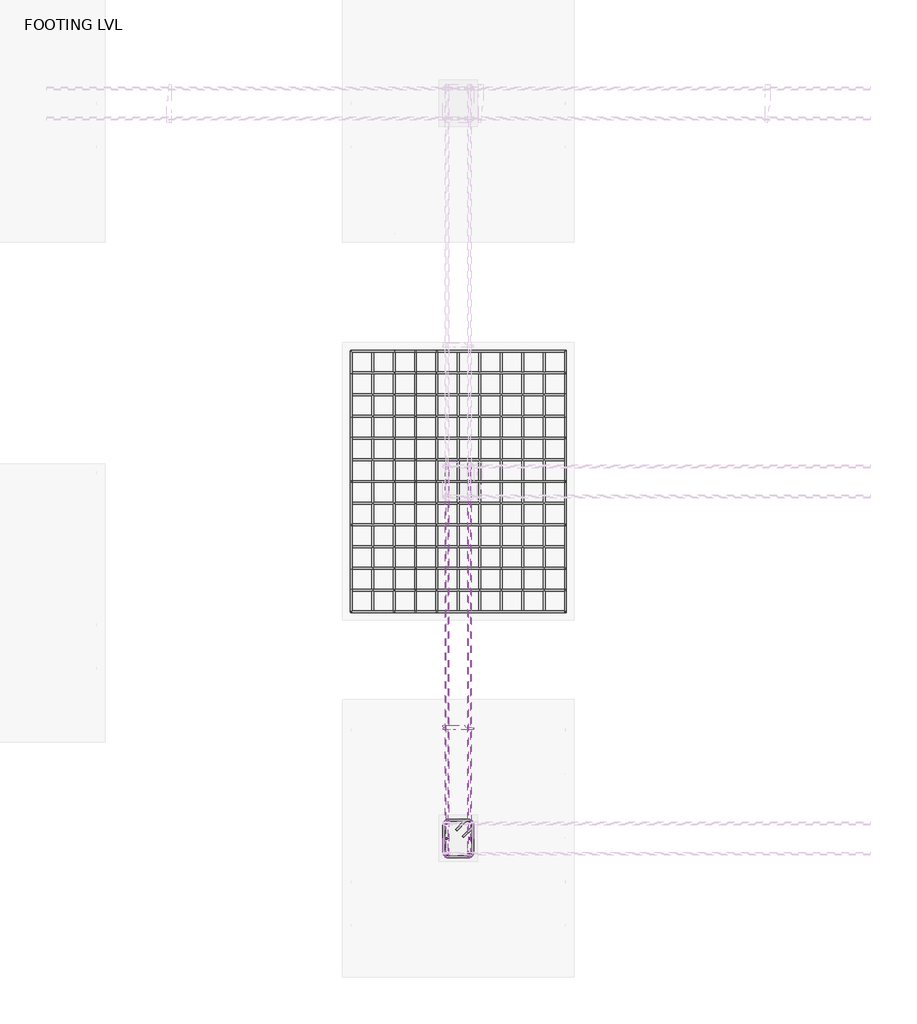
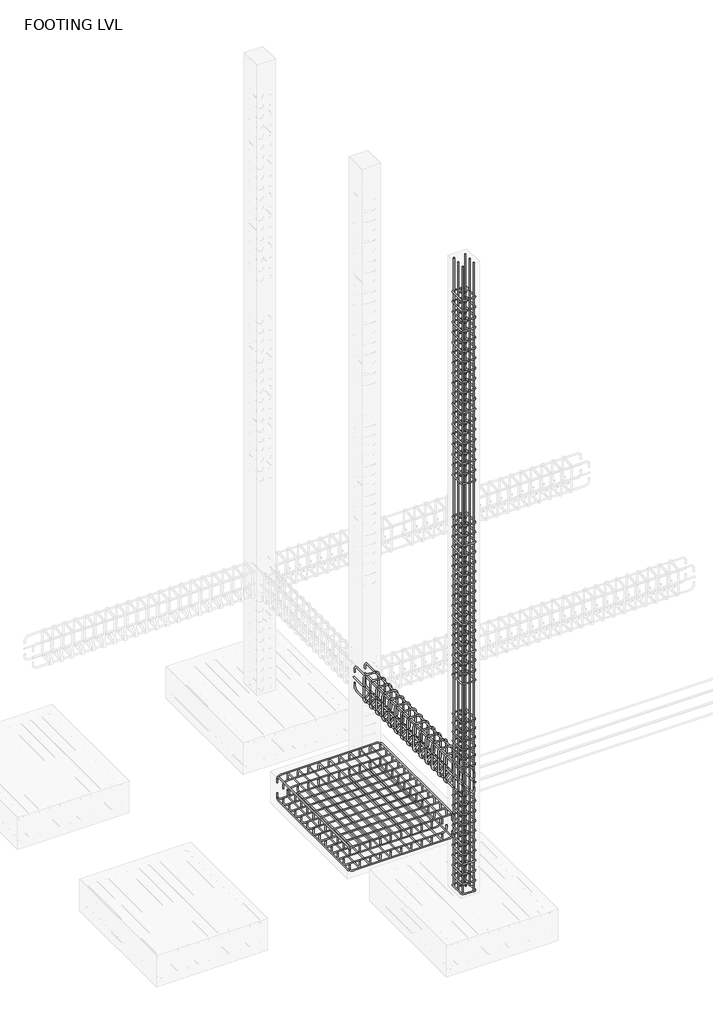
# One storey, part 3 of 16: 21 reinforcing bars.
"""IFC4 building model written with IfcOpenShell, lengths in millimetres."""

from ifc_helpers import new_model, si_unit, point, frame, origin, place, context, project, spatial, polyline, circle_curve, trimmed, segment, composite_curve, source, transform, mapped, element, save
from ifc_brep_helpers import swept_disk

model = new_model("IFC4")

# Units and contexts
model_context = context("Model", 3, world=origin())
ifc_project = project(units=[si_unit("LENGTHUNIT", "METRE", prefix="MILLI")], contexts=[model_context])

# Site, building, storey
site = spatial("IfcSite", under=ifc_project)
building = spatial("IfcBuilding", under=site)
storey = spatial("IfcBuildingStorey", under=building, Name="FOOTING LVL", Elevation=-1828.8)

# Reinforcing bars
placement = place(None, origin())
reinforcing_bar_shape = source(origin(), model_context, "Body", "SolidModel", [
    swept_disk(composite_curve([segment(polyline([(-10315.1165072, 2869.2372759, -2134.39375), (-10315.1165072, 2869.2372759, -2185.19375)]), True, "CONTINUOUS"), segment(trimmed(circle_curve(frame((-10270.6665072, 2869.2372759, -2185.19375), z_axis=(0.0, -1.0, 0.0), x_axis=(-44.45000000000073, 0.0, 0.0)), 44.45), [point((-10315.1165072, 2869.2372759, -2185.19375))], [point((-10270.6665072, 2869.2372759, -2229.64375))], True, "CARTESIAN"), True, "CONTINUOUS"), segment(polyline([(-10270.6665072, 2869.2372759, -2229.64375), (-8948.2790072, 2869.2372759, -2229.64375)]), True, "CONTINUOUS"), segment(trimmed(circle_curve(frame((-8948.2790072, 2869.2372759, -2185.19375), z_axis=(0.0, -1.0, 0.0), x_axis=(0.0, 0.0, -44.45000000000027)), 44.45), [point((-8948.2790072, 2869.2372759, -2229.64375))], [point((-8903.8290072, 2869.2372759, -2185.19375))], True, "CARTESIAN"), True, "CONTINUOUS"), segment(polyline([(-8903.8290072, 2869.2372759, -2185.19375), (-8903.8290072, 2869.2372759, -2134.39375)]), True, "CONTINUOUS")], self_intersect=False), 6.35),
])
element("IfcReinforcingBar", 1, at=placement, inside=storey, context=model_context, shape_type="MappedRepresentation", body=[
    mapped(reinforcing_bar_shape, transform((0.0, 0.0, 0.0), x_axis=(1.0, 0.0, 0.0), y_axis=(0.0, 1.0, 0.0), z_axis=(0.0, 0.0, 1.0))),
    mapped(reinforcing_bar_shape, transform((0.0, 143.0072917, 0.0), x_axis=(1.0, 0.0, 0.0), y_axis=(0.0, 1.0, 0.0), z_axis=(0.0, 0.0, 1.0))),
    mapped(reinforcing_bar_shape, transform((0.0, 286.0145833, 0.0), x_axis=(1.0, 0.0, 0.0), y_axis=(0.0, 1.0, 0.0), z_axis=(0.0, 0.0, 1.0))),
    mapped(reinforcing_bar_shape, transform((0.0, 429.021875, 0.0), x_axis=(1.0, 0.0, 0.0), y_axis=(0.0, 1.0, 0.0), z_axis=(0.0, 0.0, 1.0))),
    mapped(reinforcing_bar_shape, transform((0.0, 572.0291667, 0.0), x_axis=(1.0, 0.0, 0.0), y_axis=(0.0, 1.0, 0.0), z_axis=(0.0, 0.0, 1.0))),
    mapped(reinforcing_bar_shape, transform((0.0, 715.0364583, 0.0), x_axis=(1.0, 0.0, 0.0), y_axis=(0.0, 1.0, 0.0), z_axis=(0.0, 0.0, 1.0))),
    mapped(reinforcing_bar_shape, transform((0.0, 858.04375, 0.0), x_axis=(1.0, 0.0, 0.0), y_axis=(0.0, 1.0, 0.0), z_axis=(0.0, 0.0, 1.0))),
    mapped(reinforcing_bar_shape, transform((0.0, 1001.0510417, 0.0), x_axis=(1.0, 0.0, 0.0), y_axis=(0.0, 1.0, 0.0), z_axis=(0.0, 0.0, 1.0))),
    mapped(reinforcing_bar_shape, transform((0.0, 1144.0583333, 0.0), x_axis=(1.0, 0.0, 0.0), y_axis=(0.0, 1.0, 0.0), z_axis=(0.0, 0.0, 1.0))),
    mapped(reinforcing_bar_shape, transform((0.0, 1287.065625, 0.0), x_axis=(1.0, 0.0, 0.0), y_axis=(0.0, 1.0, 0.0), z_axis=(0.0, 0.0, 1.0))),
    mapped(reinforcing_bar_shape, transform((0.0, 1430.0729167, 0.0), x_axis=(1.0, 0.0, 0.0), y_axis=(0.0, 1.0, 0.0), z_axis=(0.0, 0.0, 1.0))),
    mapped(reinforcing_bar_shape, transform((0.0, 1573.0802083, 0.0), x_axis=(1.0, 0.0, 0.0), y_axis=(0.0, 1.0, 0.0), z_axis=(0.0, 0.0, 1.0))),
    mapped(reinforcing_bar_shape, transform((0.0, 1716.0875, 0.0), x_axis=(1.0, 0.0, 0.0), y_axis=(0.0, 1.0, 0.0), z_axis=(0.0, 0.0, 1.0))),
])
reinforcing_bar_2_shape = source(origin(), model_context, "Body", "SolidModel", [
    swept_disk(composite_curve([segment(polyline([(-8903.8290072, 2869.2372759, -1980.40625), (-8903.8290072, 2869.2372759, -1929.60625)]), True, "CONTINUOUS"), segment(trimmed(circle_curve(frame((-8948.2790072, 2869.2372759, -1929.60625), z_axis=(0.0, -1.0, 0.0), x_axis=(44.45000000000073, 0.0, 0.0)), 44.45), [point((-8903.8290072, 2869.2372759, -1929.60625))], [point((-8948.2790072, 2869.2372759, -1885.15625))], True, "CARTESIAN"), True, "CONTINUOUS"), segment(polyline([(-8948.2790072, 2869.2372759, -1885.15625), (-10270.6665072, 2869.2372759, -1885.15625)]), True, "CONTINUOUS"), segment(trimmed(circle_curve(frame((-10270.6665072, 2869.2372759, -1929.60625), z_axis=(0.0, -1.0, 0.0), x_axis=(0.0, 0.0, 44.450000000000045)), 44.45), [point((-10270.6665072, 2869.2372759, -1885.15625))], [point((-10315.1165072, 2869.2372759, -1929.60625))], True, "CARTESIAN"), True, "CONTINUOUS"), segment(polyline([(-10315.1165072, 2869.2372759, -1929.60625), (-10315.1165072, 2869.2372759, -1980.40625)]), True, "CONTINUOUS")], self_intersect=False), 6.35),
])
element("IfcReinforcingBar", 2, at=placement, inside=storey, context=model_context, shape_type="MappedRepresentation", body=[
    mapped(reinforcing_bar_2_shape, transform((0.0, 0.0, 0.0), x_axis=(1.0, 0.0, 0.0), y_axis=(0.0, 1.0, 0.0), z_axis=(0.0, 0.0, 1.0))),
    mapped(reinforcing_bar_2_shape, transform((0.0, 143.0072917, 0.0), x_axis=(1.0, 0.0, 0.0), y_axis=(0.0, 1.0, 0.0), z_axis=(0.0, 0.0, 1.0))),
    mapped(reinforcing_bar_2_shape, transform((0.0, 286.0145833, 0.0), x_axis=(1.0, 0.0, 0.0), y_axis=(0.0, 1.0, 0.0), z_axis=(0.0, 0.0, 1.0))),
    mapped(reinforcing_bar_2_shape, transform((0.0, 429.021875, 0.0), x_axis=(1.0, 0.0, 0.0), y_axis=(0.0, 1.0, 0.0), z_axis=(0.0, 0.0, 1.0))),
    mapped(reinforcing_bar_2_shape, transform((0.0, 572.0291667, 0.0), x_axis=(1.0, 0.0, 0.0), y_axis=(0.0, 1.0, 0.0), z_axis=(0.0, 0.0, 1.0))),
    mapped(reinforcing_bar_2_shape, transform((0.0, 715.0364583, 0.0), x_axis=(1.0, 0.0, 0.0), y_axis=(0.0, 1.0, 0.0), z_axis=(0.0, 0.0, 1.0))),
    mapped(reinforcing_bar_2_shape, transform((0.0, 858.04375, 0.0), x_axis=(1.0, 0.0, 0.0), y_axis=(0.0, 1.0, 0.0), z_axis=(0.0, 0.0, 1.0))),
    mapped(reinforcing_bar_2_shape, transform((0.0, 1001.0510417, 0.0), x_axis=(1.0, 0.0, 0.0), y_axis=(0.0, 1.0, 0.0), z_axis=(0.0, 0.0, 1.0))),
    mapped(reinforcing_bar_2_shape, transform((0.0, 1144.0583333, 0.0), x_axis=(1.0, 0.0, 0.0), y_axis=(0.0, 1.0, 0.0), z_axis=(0.0, 0.0, 1.0))),
    mapped(reinforcing_bar_2_shape, transform((0.0, 1287.065625, 0.0), x_axis=(1.0, 0.0, 0.0), y_axis=(0.0, 1.0, 0.0), z_axis=(0.0, 0.0, 1.0))),
    mapped(reinforcing_bar_2_shape, transform((0.0, 1430.0729167, 0.0), x_axis=(1.0, 0.0, 0.0), y_axis=(0.0, 1.0, 0.0), z_axis=(0.0, 0.0, 1.0))),
    mapped(reinforcing_bar_2_shape, transform((0.0, 1573.0802083, 0.0), x_axis=(1.0, 0.0, 0.0), y_axis=(0.0, 1.0, 0.0), z_axis=(0.0, 0.0, 1.0))),
    mapped(reinforcing_bar_2_shape, transform((0.0, 1716.0875, 0.0), x_axis=(1.0, 0.0, 0.0), y_axis=(0.0, 1.0, 0.0), z_axis=(0.0, 0.0, 1.0))),
])
reinforcing_bar_3_shape = source(origin(), model_context, "Body", "SolidModel", [
    swept_disk(composite_curve([segment(polyline([(-8903.8290072, 4585.3247759, -1980.40625), (-8903.8290072, 4585.3247759, -1929.60625)]), True, "CONTINUOUS"), segment(trimmed(circle_curve(frame((-8903.8290072, 4540.8747759, -1929.60625), z_axis=(1.0, 0.0, 0.0), x_axis=(0.0, 44.44999999999982, 0.0)), 44.45), [point((-8903.8290072, 4585.3247759, -1929.60625))], [point((-8903.8290072, 4540.8747759, -1885.15625))], True, "CARTESIAN"), True, "CONTINUOUS"), segment(polyline([(-8903.8290072, 4540.8747759, -1885.15625), (-8903.8290072, 2913.6872759, -1885.15625)]), True, "CONTINUOUS"), segment(trimmed(circle_curve(frame((-8903.8290072, 2913.6872759, -1929.60625), z_axis=(1.0, 0.0, 0.0), x_axis=(0.0, 0.0, 44.450000000000045)), 44.45), [point((-8903.8290072, 2913.6872759, -1885.15625))], [point((-8903.8290072, 2869.2372759, -1929.60625))], True, "CARTESIAN"), True, "CONTINUOUS"), segment(polyline([(-8903.8290072, 2869.2372759, -1929.60625), (-8903.8290072, 2869.2372759, -1980.40625)]), True, "CONTINUOUS")], self_intersect=False), 6.35),
])
element("IfcReinforcingBar", 3, at=placement, inside=storey, context=model_context, shape_type="MappedRepresentation", body=[
    mapped(reinforcing_bar_3_shape, transform((0.0, 0.0, 0.0), x_axis=(1.0, 0.0, 0.0), y_axis=(0.0, 1.0, 0.0), z_axis=(0.0, 0.0, 1.0))),
    mapped(reinforcing_bar_3_shape, transform((-141.12875, 0.0, 0.0), x_axis=(1.0, 0.0, 0.0), y_axis=(0.0, 1.0, 0.0), z_axis=(0.0, 0.0, 1.0))),
    mapped(reinforcing_bar_3_shape, transform((-282.2575, 0.0, 0.0), x_axis=(1.0, 0.0, 0.0), y_axis=(0.0, 1.0, 0.0), z_axis=(0.0, 0.0, 1.0))),
    mapped(reinforcing_bar_3_shape, transform((-423.38625, 0.0, 0.0), x_axis=(1.0, 0.0, 0.0), y_axis=(0.0, 1.0, 0.0), z_axis=(0.0, 0.0, 1.0))),
    mapped(reinforcing_bar_3_shape, transform((-564.515, 0.0, 0.0), x_axis=(1.0, 0.0, 0.0), y_axis=(0.0, 1.0, 0.0), z_axis=(0.0, 0.0, 1.0))),
    mapped(reinforcing_bar_3_shape, transform((-705.64375, 0.0, 0.0), x_axis=(1.0, 0.0, 0.0), y_axis=(0.0, 1.0, 0.0), z_axis=(0.0, 0.0, 1.0))),
    mapped(reinforcing_bar_3_shape, transform((-846.7725, 0.0, 0.0), x_axis=(1.0, 0.0, 0.0), y_axis=(0.0, 1.0, 0.0), z_axis=(0.0, 0.0, 1.0))),
    mapped(reinforcing_bar_3_shape, transform((-987.90125, 0.0, 0.0), x_axis=(1.0, 0.0, 0.0), y_axis=(0.0, 1.0, 0.0), z_axis=(0.0, 0.0, 1.0))),
    mapped(reinforcing_bar_3_shape, transform((-1129.03, 0.0, 0.0), x_axis=(1.0, 0.0, 0.0), y_axis=(0.0, 1.0, 0.0), z_axis=(0.0, 0.0, 1.0))),
    mapped(reinforcing_bar_3_shape, transform((-1270.15875, 0.0, 0.0), x_axis=(1.0, 0.0, 0.0), y_axis=(0.0, 1.0, 0.0), z_axis=(0.0, 0.0, 1.0))),
    mapped(reinforcing_bar_3_shape, transform((-1411.2875, 0.0, 0.0), x_axis=(1.0, 0.0, 0.0), y_axis=(0.0, 1.0, 0.0), z_axis=(0.0, 0.0, 1.0))),
])
reinforcing_bar_4_shape = source(origin(), model_context, "Body", "SolidModel", [
    swept_disk(composite_curve([segment(polyline([(-10315.1165072, 4585.3247759, -2134.39375), (-10315.1165072, 4585.3247759, -2185.19375)]), True, "CONTINUOUS"), segment(trimmed(circle_curve(frame((-10315.1165072, 4540.8747759, -2185.19375), z_axis=(-1.0, 0.0, 0.0), x_axis=(0.0, 44.44999999999982, 0.0)), 44.45), [point((-10315.1165072, 4585.3247759, -2185.19375))], [point((-10315.1165072, 4540.8747759, -2229.64375))], True, "CARTESIAN"), True, "CONTINUOUS"), segment(polyline([(-10315.1165072, 4540.8747759, -2229.64375), (-10315.1165072, 2913.6872759, -2229.64375)]), True, "CONTINUOUS"), segment(trimmed(circle_curve(frame((-10315.1165072, 2913.6872759, -2185.19375), z_axis=(-1.0, 0.0, 0.0), x_axis=(0.0, 0.0, -44.45000000000027)), 44.45), [point((-10315.1165072, 2913.6872759, -2229.64375))], [point((-10315.1165072, 2869.2372759, -2185.19375))], True, "CARTESIAN"), True, "CONTINUOUS"), segment(polyline([(-10315.1165072, 2869.2372759, -2185.19375), (-10315.1165072, 2869.2372759, -2134.39375)]), True, "CONTINUOUS")], self_intersect=False), 6.35),
])
element("IfcReinforcingBar", 4, at=placement, inside=storey, context=model_context, shape_type="MappedRepresentation", body=[
    mapped(reinforcing_bar_4_shape, transform((0.0, 0.0, 0.0), x_axis=(1.0, 0.0, 0.0), y_axis=(0.0, 1.0, 0.0), z_axis=(0.0, 0.0, 1.0))),
    mapped(reinforcing_bar_4_shape, transform((141.12875, 0.0, 0.0), x_axis=(1.0, 0.0, 0.0), y_axis=(0.0, 1.0, 0.0), z_axis=(0.0, 0.0, 1.0))),
    mapped(reinforcing_bar_4_shape, transform((282.2575, 0.0, 0.0), x_axis=(1.0, 0.0, 0.0), y_axis=(0.0, 1.0, 0.0), z_axis=(0.0, 0.0, 1.0))),
    mapped(reinforcing_bar_4_shape, transform((423.38625, 0.0, 0.0), x_axis=(1.0, 0.0, 0.0), y_axis=(0.0, 1.0, 0.0), z_axis=(0.0, 0.0, 1.0))),
    mapped(reinforcing_bar_4_shape, transform((564.515, 0.0, 0.0), x_axis=(1.0, 0.0, 0.0), y_axis=(0.0, 1.0, 0.0), z_axis=(0.0, 0.0, 1.0))),
    mapped(reinforcing_bar_4_shape, transform((705.64375, 0.0, 0.0), x_axis=(1.0, 0.0, 0.0), y_axis=(0.0, 1.0, 0.0), z_axis=(0.0, 0.0, 1.0))),
    mapped(reinforcing_bar_4_shape, transform((846.7725, 0.0, 0.0), x_axis=(1.0, 0.0, 0.0), y_axis=(0.0, 1.0, 0.0), z_axis=(0.0, 0.0, 1.0))),
    mapped(reinforcing_bar_4_shape, transform((987.90125, 0.0, 0.0), x_axis=(1.0, 0.0, 0.0), y_axis=(0.0, 1.0, 0.0), z_axis=(0.0, 0.0, 1.0))),
    mapped(reinforcing_bar_4_shape, transform((1129.03, 0.0, 0.0), x_axis=(1.0, 0.0, 0.0), y_axis=(0.0, 1.0, 0.0), z_axis=(0.0, 0.0, 1.0))),
    mapped(reinforcing_bar_4_shape, transform((1270.15875, 0.0, 0.0), x_axis=(1.0, 0.0, 0.0), y_axis=(0.0, 1.0, 0.0), z_axis=(0.0, 0.0, 1.0))),
    mapped(reinforcing_bar_4_shape, transform((1411.2875, 0.0, 0.0), x_axis=(1.0, 0.0, 0.0), y_axis=(0.0, 1.0, 0.0), z_axis=(0.0, 0.0, 1.0))),
])
reinforcing_bar_5_shape = source(origin(), model_context, "Body", "SolidModel", [
    swept_disk(composite_curve([segment(polyline([(-9625.5717485, 3568.5310259, -290.1723906), (-9691.9079326, 3568.5310259, -356.5085746)]), True, "CONTINUOUS"), segment(trimmed(circle_curve(frame((-9663.8446322, 3568.5310259, -384.571875), z_axis=(0.0, -1.0, 0.0), x_axis=(-28.063300399999207, 0.0, 28.063300400000003)), 39.6875), [point((-9691.9079326, 3568.5310259, -356.5085746))], [point((-9663.8446322, 3568.5310259, -424.259375))], True, "CARTESIAN"), True, "CONTINUOUS"), segment(polyline([(-9663.8446322, 3568.5310259, -424.259375), (-9555.1008822, 3568.5310259, -424.259375)]), True, "CONTINUOUS"), segment(trimmed(circle_curve(frame((-9555.1008822, 3568.5310259, -384.571875), z_axis=(0.0, -1.0, 0.0), x_axis=(0.0, 0.0, -39.6875)), 39.6875), [point((-9555.1008822, 3568.5310259, -424.259375))], [point((-9515.4133822, 3568.5310259, -384.571875))], True, "CARTESIAN"), True, "CONTINUOUS"), segment(polyline([(-9515.4133822, 3568.5310259, -384.571875), (-9515.4133822, 3568.5310259, -72.628125)]), True, "CONTINUOUS"), segment(trimmed(circle_curve(frame((-9554.9603179, 3571.8683201, -72.628125), z_axis=(-0.08408930148474833, -0.9964582225943078, 0.0), x_axis=(39.546935700000176, -3.3372942000000876, 0.0)), 39.6875), [point((-9515.4133822, 3568.5310259, -72.628125))], [point((-9554.9603179, 3571.8683201, -32.940625))], True, "CARTESIAN"), True, "CONTINUOUS"), segment(polyline([(-9554.9603179, 3571.8683201, -32.940625), (-9663.9851965, 3581.0687317, -32.940625)]), True, "CONTINUOUS"), segment(trimmed(circle_curve(frame((-9663.9851965, 3581.0687317, -72.628125), z_axis=(-0.08408930148474833, -0.9964582225943078, 0.0), x_axis=(0.0, 0.0, 39.6875)), 39.6875), [point((-9663.9851965, 3581.0687317, -32.940625))], [point((-9703.5321322, 3584.4060259, -72.628125))], True, "CARTESIAN"), True, "CONTINUOUS"), segment(polyline([(-9703.5321322, 3584.4060259, -72.628125), (-9703.5321322, 3584.4060259, -384.571875)]), True, "CONTINUOUS"), segment(trimmed(circle_curve(frame((-9663.8446322, 3584.4060259, -384.571875), z_axis=(0.0, -1.0, 0.0), x_axis=(-39.6875, 0.0, 0.0)), 39.6875), [point((-9703.5321322, 3584.4060259, -384.571875))], [point((-9635.7813318, 3584.4060259, -412.6351754))], True, "CARTESIAN"), True, "CONTINUOUS"), segment(polyline([(-9635.7813318, 3584.4060259, -412.6351754), (-9569.4451478, 3584.4060259, -346.2989913)]), True, "CONTINUOUS")], self_intersect=False), 7.9375),
])
element("IfcReinforcingBar", 5, at=placement, inside=storey, context=model_context, shape_type="MappedRepresentation", body=[
    mapped(reinforcing_bar_5_shape, transform((0.0, 0.0, 0.0), x_axis=(1.0, 0.0, 0.0), y_axis=(0.0, 1.0, 0.0), z_axis=(0.0, 0.0, 1.0))),
    mapped(reinforcing_bar_5_shape, transform((0.0, -146.9562281, 0.0), x_axis=(1.0, 0.0, 0.0), y_axis=(0.0, 1.0, 0.0), z_axis=(0.0, 0.0, 1.0))),
    mapped(reinforcing_bar_5_shape, transform((0.0, -293.9124561, 0.0), x_axis=(1.0, 0.0, 0.0), y_axis=(0.0, 1.0, 0.0), z_axis=(0.0, 0.0, 1.0))),
    mapped(reinforcing_bar_5_shape, transform((0.0, -440.8686842, 0.0), x_axis=(1.0, 0.0, 0.0), y_axis=(0.0, 1.0, 0.0), z_axis=(0.0, 0.0, 1.0))),
    mapped(reinforcing_bar_5_shape, transform((0.0, -587.8249123, 0.0), x_axis=(1.0, 0.0, 0.0), y_axis=(0.0, 1.0, 0.0), z_axis=(0.0, 0.0, 1.0))),
    mapped(reinforcing_bar_5_shape, transform((0.0, -734.7811403, 0.0), x_axis=(1.0, 0.0, 0.0), y_axis=(0.0, 1.0, 0.0), z_axis=(0.0, 0.0, 1.0))),
    mapped(reinforcing_bar_5_shape, transform((0.0, -881.7373684, 0.0), x_axis=(1.0, 0.0, 0.0), y_axis=(0.0, 1.0, 0.0), z_axis=(0.0, 0.0, 1.0))),
    mapped(reinforcing_bar_5_shape, transform((0.0, -1028.6935965, 0.0), x_axis=(1.0, 0.0, 0.0), y_axis=(0.0, 1.0, 0.0), z_axis=(0.0, 0.0, 1.0))),
    mapped(reinforcing_bar_5_shape, transform((0.0, -1175.6498245, 0.0), x_axis=(1.0, 0.0, 0.0), y_axis=(0.0, 1.0, 0.0), z_axis=(0.0, 0.0, 1.0))),
    mapped(reinforcing_bar_5_shape, transform((0.0, -1322.6060526, 0.0), x_axis=(1.0, 0.0, 0.0), y_axis=(0.0, 1.0, 0.0), z_axis=(0.0, 0.0, 1.0))),
    mapped(reinforcing_bar_5_shape, transform((0.0, -1469.5622806, 0.0), x_axis=(1.0, 0.0, 0.0), y_axis=(0.0, 1.0, 0.0), z_axis=(0.0, 0.0, 1.0))),
    mapped(reinforcing_bar_5_shape, transform((0.0, -1616.5185087, 0.0), x_axis=(1.0, 0.0, 0.0), y_axis=(0.0, 1.0, 0.0), z_axis=(0.0, 0.0, 1.0))),
    mapped(reinforcing_bar_5_shape, transform((0.0, -1763.4747368, 0.0), x_axis=(1.0, 0.0, 0.0), y_axis=(0.0, 1.0, 0.0), z_axis=(0.0, 0.0, 1.0))),
    mapped(reinforcing_bar_5_shape, transform((0.0, -1910.4309648, 0.0), x_axis=(1.0, 0.0, 0.0), y_axis=(0.0, 1.0, 0.0), z_axis=(0.0, 0.0, 1.0))),
])
element("IfcReinforcingBar", 6, at=placement, inside=storey, context=model_context, shape_type="SolidModel", body=[
    swept_disk(composite_curve([segment(polyline([(-9680.6826124, 3846.7404009, -307.7473552), (-9680.6826124, 3846.7404009, -345.8473552)]), True, "CONTINUOUS"), segment(trimmed(circle_curve(frame((-9680.6826124, 3791.1779009, -345.8473552), z_axis=(-1.0, 0.0, 0.0), x_axis=(0.0, 55.5625, 0.0)), 55.5625), [point((-9680.6826124, 3846.7404009, -345.8473552))], [point((-9680.6826124, 3791.1779009, -401.4098552))], True, "CARTESIAN"), True, "CONTINUOUS"), segment(polyline([(-9680.6826124, 3791.1779009, -401.4098552), (-9680.6826124, 1312.0845019, -401.4098552)]), True, "CONTINUOUS"), segment(trimmed(circle_curve(frame((-9680.6826124, 1312.0845019, -345.8473552), z_axis=(-1.0, 0.0, 0.0), x_axis=(0.0, 0.0, -55.5625)), 55.5625), [point((-9680.6826124, 1312.0845019, -401.4098552))], [point((-9680.6826124, 1256.5220019, -345.8473552))], True, "CARTESIAN"), True, "CONTINUOUS"), segment(polyline([(-9680.6826124, 1256.5220019, -345.8473552), (-9680.6826124, 1256.5220019, -307.7473552)]), True, "CONTINUOUS")], self_intersect=False), 7.9375),
])
element("IfcReinforcingBar", 7, at=placement, inside=storey, context=model_context, shape_type="SolidModel", body=[
    swept_disk(composite_curve([segment(polyline([(-9538.262902, 3846.7404009, -307.7473552), (-9538.262902, 3846.7404009, -345.8473552)]), True, "CONTINUOUS"), segment(trimmed(circle_curve(frame((-9538.262902, 3791.1779009, -345.8473552), z_axis=(-1.0, 0.0, 0.0), x_axis=(0.0, 55.5625, 0.0)), 55.5625), [point((-9538.262902, 3846.7404009, -345.8473552))], [point((-9538.262902, 3791.1779009, -401.4098552))], True, "CARTESIAN"), True, "CONTINUOUS"), segment(polyline([(-9538.262902, 3791.1779009, -401.4098552), (-9538.262902, 1312.0845019, -401.4098552)]), True, "CONTINUOUS"), segment(trimmed(circle_curve(frame((-9538.262902, 1312.0845019, -345.8473552), z_axis=(-1.0, 0.0, 0.0), x_axis=(0.0, 0.0, -55.5625)), 55.5625), [point((-9538.262902, 1312.0845019, -401.4098552))], [point((-9538.262902, 1256.5220019, -345.8473552))], True, "CARTESIAN"), True, "CONTINUOUS"), segment(polyline([(-9538.262902, 1256.5220019, -345.8473552), (-9538.262902, 1256.5220019, -307.7473552)]), True, "CONTINUOUS")], self_intersect=False), 7.9375),
])
element("IfcReinforcingBar", 8, at=placement, inside=storey, context=model_context, shape_type="SolidModel", body=[
    swept_disk(composite_curve([segment(polyline([(-9680.6826124, 3846.7404009, -149.4526448), (-9680.6826124, 3846.7404009, -111.3526448)]), True, "CONTINUOUS"), segment(trimmed(circle_curve(frame((-9680.6826124, 3791.1779009, -111.3526448), z_axis=(1.0, 0.0, 0.0), x_axis=(0.0, 55.5625, 0.0)), 55.5625), [point((-9680.6826124, 3846.7404009, -111.3526448))], [point((-9680.6826124, 3791.1779009, -55.7901448))], True, "CARTESIAN"), True, "CONTINUOUS"), segment(polyline([(-9680.6826124, 3791.1779009, -55.7901448), (-9680.6826124, 1312.0845019, -55.7901448)]), True, "CONTINUOUS"), segment(trimmed(circle_curve(frame((-9680.6826124, 1312.0845019, -111.3526448), z_axis=(1.0, 0.0, 0.0), x_axis=(0.0, 0.0, 55.56249999999999)), 55.5625), [point((-9680.6826124, 1312.0845019, -55.7901448))], [point((-9680.6826124, 1256.5220019, -111.3526448))], True, "CARTESIAN"), True, "CONTINUOUS"), segment(polyline([(-9680.6826124, 1256.5220019, -111.3526448), (-9680.6826124, 1256.5220019, -149.4526448)]), True, "CONTINUOUS")], self_intersect=False), 7.9375),
])
element("IfcReinforcingBar", 9, at=placement, inside=storey, context=model_context, shape_type="SolidModel", body=[
    swept_disk(composite_curve([segment(polyline([(-9538.262902, 3846.7404009, -149.4526448), (-9538.262902, 3846.7404009, -111.3526448)]), True, "CONTINUOUS"), segment(trimmed(circle_curve(frame((-9538.262902, 3791.1779009, -111.3526448), z_axis=(1.0, 0.0, 0.0), x_axis=(0.0, 55.5625, 0.0)), 55.5625), [point((-9538.262902, 3846.7404009, -111.3526448))], [point((-9538.262902, 3791.1779009, -55.7901448))], True, "CARTESIAN"), True, "CONTINUOUS"), segment(polyline([(-9538.262902, 3791.1779009, -55.7901448), (-9538.262902, 1312.0845019, -55.7901448)]), True, "CONTINUOUS"), segment(trimmed(circle_curve(frame((-9538.262902, 1312.0845019, -111.3526448), z_axis=(1.0, 0.0, 0.0), x_axis=(0.0, 0.0, 55.56249999999999)), 55.5625), [point((-9538.262902, 1312.0845019, -55.7901448))], [point((-9538.262902, 1256.5220019, -111.3526448))], True, "CARTESIAN"), True, "CONTINUOUS"), segment(polyline([(-9538.262902, 1256.5220019, -111.3526448), (-9538.262902, 1256.5220019, -149.4526448)]), True, "CONTINUOUS")], self_intersect=False), 7.9375),
])
element("IfcReinforcingBar", 10, at=placement, inside=storey, context=model_context, shape_type="SolidModel", body=[
    swept_disk(composite_curve([segment(polyline([(-9686.8400164, 3854.6779009, -228.6), (-9686.8400164, 1248.5845019, -228.6)]), True, "CONTINUOUS")], self_intersect=False), 7.9375),
])
element("IfcReinforcingBar", 11, at=placement, inside=storey, context=model_context, shape_type="SolidModel", body=[
    swept_disk(composite_curve([segment(polyline([(-9532.105498, 3854.6779009, -228.6), (-9532.105498, 1248.5845019, -228.6)]), True, "CONTINUOUS")], self_intersect=False), 7.9375),
])
reinforcing_bar_6_shape = source(origin(), model_context, "Body", "SolidModel", [
    swept_disk(composite_curve([segment(polyline([(-9577.9902404, 1387.9626131, -1797.446875), (-9523.1252419, 1442.8276116, -1797.446875)]), True, "CONTINUOUS"), segment(trimmed(circle_curve(frame((-9545.5758822, 1465.2782519, -1797.446875), z_axis=(0.0, 0.0, 1.0), x_axis=(22.450640300001396, -22.450640300000032, 0.0)), 31.75), [point((-9523.1252419, 1442.8276116, -1797.446875))], [point((-9545.5758822, 1497.0282519, -1797.446875))], True, "CARTESIAN"), True, "CONTINUOUS"), segment(polyline([(-9545.5758822, 1497.0282519, -1797.446875), (-9673.3696322, 1497.0282519, -1797.446875)]), True, "CONTINUOUS"), segment(trimmed(circle_curve(frame((-9673.3696322, 1465.2782519, -1797.446875), z_axis=(0.0, 0.0, 1.0), x_axis=(0.0, 31.75, 0.0)), 31.75), [point((-9673.3696322, 1497.0282519, -1797.446875))], [point((-9705.1196322, 1465.2782519, -1797.446875))], True, "CARTESIAN"), True, "CONTINUOUS"), segment(polyline([(-9705.1196322, 1465.2782519, -1797.446875), (-9705.1196322, 1286.6845019, -1797.446875)]), True, "CONTINUOUS"), segment(trimmed(circle_curve(frame((-9673.439373, 1286.6845019, -1799.5501287), z_axis=(0.06624421176864072, 0.0, 0.9978034397651431), x_axis=(-31.680259200000364, 0.0, 2.1032536999998683)), 31.75), [point((-9705.1196322, 1286.6845019, -1797.446875))], [point((-9673.439373, 1254.9345019, -1799.5501287))], True, "CARTESIAN"), True, "CONTINUOUS"), segment(polyline([(-9673.439373, 1254.9345019, -1799.5501287), (-9545.5061414, 1254.9345019, -1808.0436213)]), True, "CONTINUOUS"), segment(trimmed(circle_curve(frame((-9545.5061414, 1286.6845019, -1808.0436213), z_axis=(0.06624421176864072, 0.0, 0.9978034397651431), x_axis=(0.0, -31.75, 0.0)), 31.75), [point((-9545.5061414, 1254.9345019, -1808.0436213))], [point((-9513.8258822, 1286.6845019, -1810.146875))], True, "CARTESIAN"), True, "CONTINUOUS"), segment(polyline([(-9513.8258822, 1286.6845019, -1810.146875), (-9513.8258822, 1465.2782519, -1810.146875)]), True, "CONTINUOUS"), segment(trimmed(circle_curve(frame((-9545.5758822, 1465.2782519, -1810.146875), z_axis=(0.0, 0.0, 1.0), x_axis=(31.75, 0.0, 0.0)), 31.75), [point((-9513.8258822, 1465.2782519, -1810.146875))], [point((-9568.0265225, 1487.7288922, -1810.146875))], True, "CARTESIAN"), True, "CONTINUOUS"), segment(polyline([(-9568.0265225, 1487.7288922, -1810.146875), (-9622.891521, 1432.8638937, -1810.146875)]), True, "CONTINUOUS")], self_intersect=False), 6.35),
])
element("IfcReinforcingBar", 12, at=placement, inside=storey, context=model_context, shape_type="MappedRepresentation", body=[
    mapped(reinforcing_bar_6_shape, transform((0.0, 0.0, 0.0), x_axis=(1.0, 0.0, 0.0), y_axis=(0.0, 1.0, 0.0), z_axis=(0.0, 0.0, 1.0))),
    mapped(reinforcing_bar_6_shape, transform((0.0, 0.0, 144.2276574), x_axis=(1.0, 0.0, 0.0), y_axis=(0.0, 1.0, 0.0), z_axis=(0.0, 0.0, 1.0))),
    mapped(reinforcing_bar_6_shape, transform((0.0, 0.0, 288.4553149), x_axis=(1.0, 0.0, 0.0), y_axis=(0.0, 1.0, 0.0), z_axis=(0.0, 0.0, 1.0))),
    mapped(reinforcing_bar_6_shape, transform((0.0, 0.0, 432.6829723), x_axis=(1.0, 0.0, 0.0), y_axis=(0.0, 1.0, 0.0), z_axis=(0.0, 0.0, 1.0))),
    mapped(reinforcing_bar_6_shape, transform((0.0, 0.0, 576.9106298), x_axis=(1.0, 0.0, 0.0), y_axis=(0.0, 1.0, 0.0), z_axis=(0.0, 0.0, 1.0))),
    mapped(reinforcing_bar_6_shape, transform((0.0, 0.0, 721.1382872), x_axis=(1.0, 0.0, 0.0), y_axis=(0.0, 1.0, 0.0), z_axis=(0.0, 0.0, 1.0))),
    mapped(reinforcing_bar_6_shape, transform((0.0, 0.0, 865.3659446), x_axis=(1.0, 0.0, 0.0), y_axis=(0.0, 1.0, 0.0), z_axis=(0.0, 0.0, 1.0))),
    mapped(reinforcing_bar_6_shape, transform((0.0, 0.0, 1009.5936021), x_axis=(1.0, 0.0, 0.0), y_axis=(0.0, 1.0, 0.0), z_axis=(0.0, 0.0, 1.0))),
    mapped(reinforcing_bar_6_shape, transform((0.0, 0.0, 1153.8212595), x_axis=(1.0, 0.0, 0.0), y_axis=(0.0, 1.0, 0.0), z_axis=(0.0, 0.0, 1.0))),
    mapped(reinforcing_bar_6_shape, transform((0.0, 0.0, 1298.048917), x_axis=(1.0, 0.0, 0.0), y_axis=(0.0, 1.0, 0.0), z_axis=(0.0, 0.0, 1.0))),
])
element("IfcReinforcingBar", 13, at=placement, inside=storey, context=model_context, shape_type="SolidModel", body=[
    swept_disk(composite_curve([segment(polyline([(-9532.105498, 1478.7486361, -1803.796875), (-9532.105498, 1478.7486361, 7290.196875)]), True, "CONTINUOUS")], self_intersect=False), 6.35),
])
element("IfcReinforcingBar", 14, at=placement, inside=storey, context=model_context, shape_type="SolidModel", body=[
    swept_disk(composite_curve([segment(polyline([(-9686.8400164, 1478.7486361, -1803.796875), (-9686.8400164, 1478.7486361, 7290.196875)]), True, "CONTINUOUS")], self_intersect=False), 6.35),
])
element("IfcReinforcingBar", 15, at=placement, inside=storey, context=model_context, shape_type="SolidModel", body=[
    swept_disk(composite_curve([segment(polyline([(-9532.105498, 1273.2141177, -1803.796875), (-9532.105498, 1273.2141177, 7290.196875)]), True, "CONTINUOUS")], self_intersect=False), 6.35),
])
element("IfcReinforcingBar", 16, at=placement, inside=storey, context=model_context, shape_type="SolidModel", body=[
    swept_disk(composite_curve([segment(polyline([(-9686.8400164, 1273.2141177, -1803.796875), (-9686.8400164, 1273.2141177, 7290.196875)]), True, "CONTINUOUS")], self_intersect=False), 6.35),
])
element("IfcReinforcingBar", 17, at=placement, inside=storey, context=model_context, shape_type="SolidModel", body=[
    swept_disk(composite_curve([segment(polyline([(-9532.105498, 1375.9813769, -1803.796875), (-9532.105498, 1375.9813769, 7290.196875)]), True, "CONTINUOUS")], self_intersect=False), 6.35),
])
element("IfcReinforcingBar", 18, at=placement, inside=storey, context=model_context, shape_type="SolidModel", body=[
    swept_disk(composite_curve([segment(polyline([(-9686.8400164, 1375.9813769, -1803.796875), (-9686.8400164, 1375.9813769, 7290.196875)]), True, "CONTINUOUS")], self_intersect=False), 6.35),
])
reinforcing_bar_7_shape = source(origin(), model_context, "Body", "SolidModel", [
    swept_disk(composite_curve([segment(polyline([(-9577.9902404, 1387.9626131, 31.353125), (-9523.1252419, 1442.8276116, 31.353125)]), True, "CONTINUOUS"), segment(trimmed(circle_curve(frame((-9545.5758822, 1465.2782519, 31.353125), z_axis=(0.0, 0.0, 1.0), x_axis=(22.450640300001396, -22.450640300000032, 0.0)), 31.75), [point((-9523.1252419, 1442.8276116, 31.353125))], [point((-9545.5758822, 1497.0282519, 31.353125))], True, "CARTESIAN"), True, "CONTINUOUS"), segment(polyline([(-9545.5758822, 1497.0282519, 31.353125), (-9673.3696322, 1497.0282519, 31.353125)]), True, "CONTINUOUS"), segment(trimmed(circle_curve(frame((-9673.3696322, 1465.2782519, 31.353125), z_axis=(0.0, 0.0, 1.0), x_axis=(0.0, 31.75, 0.0)), 31.75), [point((-9673.3696322, 1497.0282519, 31.353125))], [point((-9705.1196322, 1465.2782519, 31.353125))], True, "CARTESIAN"), True, "CONTINUOUS"), segment(polyline([(-9705.1196322, 1465.2782519, 31.353125), (-9705.1196322, 1286.6845019, 31.353125)]), True, "CONTINUOUS"), segment(trimmed(circle_curve(frame((-9673.439373, 1286.6845019, 29.2498713), z_axis=(0.06624421176864072, 0.0, 0.9978034397651431), x_axis=(-31.680259200000364, 0.0, 2.1032537)), 31.75), [point((-9705.1196322, 1286.6845019, 31.353125))], [point((-9673.439373, 1254.9345019, 29.2498713))], True, "CARTESIAN"), True, "CONTINUOUS"), segment(polyline([(-9673.439373, 1254.9345019, 29.2498713), (-9545.5061414, 1254.9345019, 20.7563787)]), True, "CONTINUOUS"), segment(trimmed(circle_curve(frame((-9545.5061414, 1286.6845019, 20.7563787), z_axis=(0.06624421176864072, 0.0, 0.9978034397651431), x_axis=(0.0, -31.75, 0.0)), 31.75), [point((-9545.5061414, 1254.9345019, 20.7563787))], [point((-9513.8258822, 1286.6845019, 18.653125))], True, "CARTESIAN"), True, "CONTINUOUS"), segment(polyline([(-9513.8258822, 1286.6845019, 18.653125), (-9513.8258822, 1465.2782519, 18.653125)]), True, "CONTINUOUS"), segment(trimmed(circle_curve(frame((-9545.5758822, 1465.2782519, 18.653125), z_axis=(0.0, 0.0, 1.0), x_axis=(31.75, 0.0, 0.0)), 31.75), [point((-9513.8258822, 1465.2782519, 18.653125))], [point((-9568.0265225, 1487.7288922, 18.653125))], True, "CARTESIAN"), True, "CONTINUOUS"), segment(polyline([(-9568.0265225, 1487.7288922, 18.653125), (-9622.891521, 1432.8638937, 18.653125)]), True, "CONTINUOUS")], self_intersect=False), 6.35),
])
element("IfcReinforcingBar", 19, at=placement, inside=storey, context=model_context, shape_type="MappedRepresentation", body=[
    mapped(reinforcing_bar_7_shape, transform((0.0, 0.0, 0.0), x_axis=(1.0, 0.0, 0.0), y_axis=(0.0, 1.0, 0.0), z_axis=(0.0, 0.0, 1.0))),
    mapped(reinforcing_bar_7_shape, transform((0.0, 0.0, 130.6477176), x_axis=(1.0, 0.0, 0.0), y_axis=(0.0, 1.0, 0.0), z_axis=(0.0, 0.0, 1.0))),
    mapped(reinforcing_bar_7_shape, transform((0.0, 0.0, 261.2954352), x_axis=(1.0, 0.0, 0.0), y_axis=(0.0, 1.0, 0.0), z_axis=(0.0, 0.0, 1.0))),
    mapped(reinforcing_bar_7_shape, transform((0.0, 0.0, 391.9431528), x_axis=(1.0, 0.0, 0.0), y_axis=(0.0, 1.0, 0.0), z_axis=(0.0, 0.0, 1.0))),
    mapped(reinforcing_bar_7_shape, transform((0.0, 0.0, 522.5908704), x_axis=(1.0, 0.0, 0.0), y_axis=(0.0, 1.0, 0.0), z_axis=(0.0, 0.0, 1.0))),
    mapped(reinforcing_bar_7_shape, transform((0.0, 0.0, 653.238588), x_axis=(1.0, 0.0, 0.0), y_axis=(0.0, 1.0, 0.0), z_axis=(0.0, 0.0, 1.0))),
])
reinforcing_bar_8_shape = source(origin(), model_context, "Body", "SolidModel", [
    swept_disk(composite_curve([segment(polyline([(-9577.9902404, 1387.9626131, 1250.553125), (-9523.1252419, 1442.8276116, 1250.553125)]), True, "CONTINUOUS"), segment(trimmed(circle_curve(frame((-9545.5758822, 1465.2782519, 1250.553125), z_axis=(0.0, 0.0, 1.0), x_axis=(22.450640300001396, -22.450640300000032, 0.0)), 31.75), [point((-9523.1252419, 1442.8276116, 1250.553125))], [point((-9545.5758822, 1497.0282519, 1250.553125))], True, "CARTESIAN"), True, "CONTINUOUS"), segment(polyline([(-9545.5758822, 1497.0282519, 1250.553125), (-9673.3696322, 1497.0282519, 1250.553125)]), True, "CONTINUOUS"), segment(trimmed(circle_curve(frame((-9673.3696322, 1465.2782519, 1250.553125), z_axis=(0.0, 0.0, 1.0), x_axis=(0.0, 31.75, 0.0)), 31.75), [point((-9673.3696322, 1497.0282519, 1250.553125))], [point((-9705.1196322, 1465.2782519, 1250.553125))], True, "CARTESIAN"), True, "CONTINUOUS"), segment(polyline([(-9705.1196322, 1465.2782519, 1250.553125), (-9705.1196322, 1286.6845019, 1250.553125)]), True, "CONTINUOUS"), segment(trimmed(circle_curve(frame((-9673.439373, 1286.6845019, 1248.4498713), z_axis=(0.06624421176864072, 0.0, 0.9978034397651431), x_axis=(-31.680259200000364, 0.0, 2.1032536999998683)), 31.75), [point((-9705.1196322, 1286.6845019, 1250.553125))], [point((-9673.439373, 1254.9345019, 1248.4498713))], True, "CARTESIAN"), True, "CONTINUOUS"), segment(polyline([(-9673.439373, 1254.9345019, 1248.4498713), (-9545.5061414, 1254.9345019, 1239.9563787)]), True, "CONTINUOUS"), segment(trimmed(circle_curve(frame((-9545.5061414, 1286.6845019, 1239.9563787), z_axis=(0.06624421176864072, 0.0, 0.9978034397651431), x_axis=(0.0, -31.75, 0.0)), 31.75), [point((-9545.5061414, 1254.9345019, 1239.9563787))], [point((-9513.8258822, 1286.6845019, 1237.853125))], True, "CARTESIAN"), True, "CONTINUOUS"), segment(polyline([(-9513.8258822, 1286.6845019, 1237.853125), (-9513.8258822, 1465.2782519, 1237.853125)]), True, "CONTINUOUS"), segment(trimmed(circle_curve(frame((-9545.5758822, 1465.2782519, 1237.853125), z_axis=(0.0, 0.0, 1.0), x_axis=(31.75, 0.0, 0.0)), 31.75), [point((-9513.8258822, 1465.2782519, 1237.853125))], [point((-9568.0265225, 1487.7288922, 1237.853125))], True, "CARTESIAN"), True, "CONTINUOUS"), segment(polyline([(-9568.0265225, 1487.7288922, 1237.853125), (-9622.891521, 1432.8638937, 1237.853125)]), True, "CONTINUOUS")], self_intersect=False), 6.35),
])
element("IfcReinforcingBar", 20, at=placement, inside=storey, context=model_context, shape_type="MappedRepresentation", body=[
    mapped(reinforcing_bar_8_shape, transform((0.0, 0.0, 0.0), x_axis=(1.0, 0.0, 0.0), y_axis=(0.0, 1.0, 0.0), z_axis=(0.0, 0.0, 1.0))),
    mapped(reinforcing_bar_8_shape, transform((0.0, 0.0, 142.9836687), x_axis=(1.0, 0.0, 0.0), y_axis=(0.0, 1.0, 0.0), z_axis=(0.0, 0.0, 1.0))),
    mapped(reinforcing_bar_8_shape, transform((0.0, 0.0, 285.9673374), x_axis=(1.0, 0.0, 0.0), y_axis=(0.0, 1.0, 0.0), z_axis=(0.0, 0.0, 1.0))),
    mapped(reinforcing_bar_8_shape, transform((0.0, 0.0, 428.9510061), x_axis=(1.0, 0.0, 0.0), y_axis=(0.0, 1.0, 0.0), z_axis=(0.0, 0.0, 1.0))),
    mapped(reinforcing_bar_8_shape, transform((0.0, 0.0, 571.9346748), x_axis=(1.0, 0.0, 0.0), y_axis=(0.0, 1.0, 0.0), z_axis=(0.0, 0.0, 1.0))),
    mapped(reinforcing_bar_8_shape, transform((0.0, 0.0, 714.9183435), x_axis=(1.0, 0.0, 0.0), y_axis=(0.0, 1.0, 0.0), z_axis=(0.0, 0.0, 1.0))),
    mapped(reinforcing_bar_8_shape, transform((0.0, 0.0, 857.9020122), x_axis=(1.0, 0.0, 0.0), y_axis=(0.0, 1.0, 0.0), z_axis=(0.0, 0.0, 1.0))),
    mapped(reinforcing_bar_8_shape, transform((0.0, 0.0, 1000.8856809), x_axis=(1.0, 0.0, 0.0), y_axis=(0.0, 1.0, 0.0), z_axis=(0.0, 0.0, 1.0))),
    mapped(reinforcing_bar_8_shape, transform((0.0, 0.0, 1143.8693496), x_axis=(1.0, 0.0, 0.0), y_axis=(0.0, 1.0, 0.0), z_axis=(0.0, 0.0, 1.0))),
    mapped(reinforcing_bar_8_shape, transform((0.0, 0.0, 1286.8530183), x_axis=(1.0, 0.0, 0.0), y_axis=(0.0, 1.0, 0.0), z_axis=(0.0, 0.0, 1.0))),
    mapped(reinforcing_bar_8_shape, transform((0.0, 0.0, 1429.836687), x_axis=(1.0, 0.0, 0.0), y_axis=(0.0, 1.0, 0.0), z_axis=(0.0, 0.0, 1.0))),
    mapped(reinforcing_bar_8_shape, transform((0.0, 0.0, 1572.8203557), x_axis=(1.0, 0.0, 0.0), y_axis=(0.0, 1.0, 0.0), z_axis=(0.0, 0.0, 1.0))),
    mapped(reinforcing_bar_8_shape, transform((0.0, 0.0, 1715.8040244), x_axis=(1.0, 0.0, 0.0), y_axis=(0.0, 1.0, 0.0), z_axis=(0.0, 0.0, 1.0))),
    mapped(reinforcing_bar_8_shape, transform((0.0, 0.0, 1858.7876931), x_axis=(1.0, 0.0, 0.0), y_axis=(0.0, 1.0, 0.0), z_axis=(0.0, 0.0, 1.0))),
    mapped(reinforcing_bar_8_shape, transform((0.0, 0.0, 2001.7713618), x_axis=(1.0, 0.0, 0.0), y_axis=(0.0, 1.0, 0.0), z_axis=(0.0, 0.0, 1.0))),
    mapped(reinforcing_bar_8_shape, transform((0.0, 0.0, 2144.7550305), x_axis=(1.0, 0.0, 0.0), y_axis=(0.0, 1.0, 0.0), z_axis=(0.0, 0.0, 1.0))),
    mapped(reinforcing_bar_8_shape, transform((0.0, 0.0, 2287.7386992), x_axis=(1.0, 0.0, 0.0), y_axis=(0.0, 1.0, 0.0), z_axis=(0.0, 0.0, 1.0))),
])
reinforcing_bar_9_shape = source(origin(), model_context, "Body", "SolidModel", [
    swept_disk(composite_curve([segment(polyline([(-9577.9902404, 1387.9626131, 4146.153125), (-9523.1252419, 1442.8276116, 4146.153125)]), True, "CONTINUOUS"), segment(trimmed(circle_curve(frame((-9545.5758822, 1465.2782519, 4146.153125), z_axis=(0.0, 0.0, 1.0), x_axis=(22.450640300001396, -22.450640300000032, 0.0)), 31.75), [point((-9523.1252419, 1442.8276116, 4146.153125))], [point((-9545.5758822, 1497.0282519, 4146.153125))], True, "CARTESIAN"), True, "CONTINUOUS"), segment(polyline([(-9545.5758822, 1497.0282519, 4146.153125), (-9673.3696322, 1497.0282519, 4146.153125)]), True, "CONTINUOUS"), segment(trimmed(circle_curve(frame((-9673.3696322, 1465.2782519, 4146.153125), z_axis=(0.0, 0.0, 1.0), x_axis=(0.0, 31.75, 0.0)), 31.75), [point((-9673.3696322, 1497.0282519, 4146.153125))], [point((-9705.1196322, 1465.2782519, 4146.153125))], True, "CARTESIAN"), True, "CONTINUOUS"), segment(polyline([(-9705.1196322, 1465.2782519, 4146.153125), (-9705.1196322, 1286.6845019, 4146.153125)]), True, "CONTINUOUS"), segment(trimmed(circle_curve(frame((-9673.439373, 1286.6845019, 4144.0498713), z_axis=(0.06624421176864072, 0.0, 0.9978034397651431), x_axis=(-31.680259200000364, 0.0, 2.1032537000000957)), 31.75), [point((-9705.1196322, 1286.6845019, 4146.153125))], [point((-9673.439373, 1254.9345019, 4144.0498713))], True, "CARTESIAN"), True, "CONTINUOUS"), segment(polyline([(-9673.439373, 1254.9345019, 4144.0498713), (-9545.5061414, 1254.9345019, 4135.5563787)]), True, "CONTINUOUS"), segment(trimmed(circle_curve(frame((-9545.5061414, 1286.6845019, 4135.5563787), z_axis=(0.06624421176864072, 0.0, 0.9978034397651431), x_axis=(0.0, -31.75, 0.0)), 31.75), [point((-9545.5061414, 1254.9345019, 4135.5563787))], [point((-9513.8258822, 1286.6845019, 4133.453125))], True, "CARTESIAN"), True, "CONTINUOUS"), segment(polyline([(-9513.8258822, 1286.6845019, 4133.453125), (-9513.8258822, 1465.2782519, 4133.453125)]), True, "CONTINUOUS"), segment(trimmed(circle_curve(frame((-9545.5758822, 1465.2782519, 4133.453125), z_axis=(0.0, 0.0, 1.0), x_axis=(31.75, 0.0, 0.0)), 31.75), [point((-9513.8258822, 1465.2782519, 4133.453125))], [point((-9568.0265225, 1487.7288922, 4133.453125))], True, "CARTESIAN"), True, "CONTINUOUS"), segment(polyline([(-9568.0265225, 1487.7288922, 4133.453125), (-9622.891521, 1432.8638937, 4133.453125)]), True, "CONTINUOUS")], self_intersect=False), 6.35),
])
element("IfcReinforcingBar", 21, at=placement, inside=storey, context=model_context, shape_type="MappedRepresentation", body=[
    mapped(reinforcing_bar_9_shape, transform((0.0, 0.0, 0.0), x_axis=(1.0, 0.0, 0.0), y_axis=(0.0, 1.0, 0.0), z_axis=(0.0, 0.0, 1.0))),
    mapped(reinforcing_bar_9_shape, transform((0.0, 0.0, 147.7188031), x_axis=(1.0, 0.0, 0.0), y_axis=(0.0, 1.0, 0.0), z_axis=(0.0, 0.0, 1.0))),
    mapped(reinforcing_bar_9_shape, transform((0.0, 0.0, 295.4376062), x_axis=(1.0, 0.0, 0.0), y_axis=(0.0, 1.0, 0.0), z_axis=(0.0, 0.0, 1.0))),
    mapped(reinforcing_bar_9_shape, transform((0.0, 0.0, 443.1564093), x_axis=(1.0, 0.0, 0.0), y_axis=(0.0, 1.0, 0.0), z_axis=(0.0, 0.0, 1.0))),
    mapped(reinforcing_bar_9_shape, transform((0.0, 0.0, 590.8752124), x_axis=(1.0, 0.0, 0.0), y_axis=(0.0, 1.0, 0.0), z_axis=(0.0, 0.0, 1.0))),
    mapped(reinforcing_bar_9_shape, transform((0.0, 0.0, 738.5940155), x_axis=(1.0, 0.0, 0.0), y_axis=(0.0, 1.0, 0.0), z_axis=(0.0, 0.0, 1.0))),
    mapped(reinforcing_bar_9_shape, transform((0.0, 0.0, 886.3128187), x_axis=(1.0, 0.0, 0.0), y_axis=(0.0, 1.0, 0.0), z_axis=(0.0, 0.0, 1.0))),
    mapped(reinforcing_bar_9_shape, transform((0.0, 0.0, 1034.0316218), x_axis=(1.0, 0.0, 0.0), y_axis=(0.0, 1.0, 0.0), z_axis=(0.0, 0.0, 1.0))),
    mapped(reinforcing_bar_9_shape, transform((0.0, 0.0, 1181.7504249), x_axis=(1.0, 0.0, 0.0), y_axis=(0.0, 1.0, 0.0), z_axis=(0.0, 0.0, 1.0))),
    mapped(reinforcing_bar_9_shape, transform((0.0, 0.0, 1329.469228), x_axis=(1.0, 0.0, 0.0), y_axis=(0.0, 1.0, 0.0), z_axis=(0.0, 0.0, 1.0))),
    mapped(reinforcing_bar_9_shape, transform((0.0, 0.0, 1477.1880311), x_axis=(1.0, 0.0, 0.0), y_axis=(0.0, 1.0, 0.0), z_axis=(0.0, 0.0, 1.0))),
    mapped(reinforcing_bar_9_shape, transform((0.0, 0.0, 1624.9068342), x_axis=(1.0, 0.0, 0.0), y_axis=(0.0, 1.0, 0.0), z_axis=(0.0, 0.0, 1.0))),
    mapped(reinforcing_bar_9_shape, transform((0.0, 0.0, 1772.6256373), x_axis=(1.0, 0.0, 0.0), y_axis=(0.0, 1.0, 0.0), z_axis=(0.0, 0.0, 1.0))),
    mapped(reinforcing_bar_9_shape, transform((0.0, 0.0, 1920.3444404), x_axis=(1.0, 0.0, 0.0), y_axis=(0.0, 1.0, 0.0), z_axis=(0.0, 0.0, 1.0))),
    mapped(reinforcing_bar_9_shape, transform((0.0, 0.0, 2068.0632435), x_axis=(1.0, 0.0, 0.0), y_axis=(0.0, 1.0, 0.0), z_axis=(0.0, 0.0, 1.0))),
    mapped(reinforcing_bar_9_shape, transform((0.0, 0.0, 2215.7820466), x_axis=(1.0, 0.0, 0.0), y_axis=(0.0, 1.0, 0.0), z_axis=(0.0, 0.0, 1.0))),
    mapped(reinforcing_bar_9_shape, transform((0.0, 0.0, 2363.5008497), x_axis=(1.0, 0.0, 0.0), y_axis=(0.0, 1.0, 0.0), z_axis=(0.0, 0.0, 1.0))),
    mapped(reinforcing_bar_9_shape, transform((0.0, 0.0, 2511.2196529), x_axis=(1.0, 0.0, 0.0), y_axis=(0.0, 1.0, 0.0), z_axis=(0.0, 0.0, 1.0))),
    mapped(reinforcing_bar_9_shape, transform((0.0, 0.0, 2658.938456), x_axis=(1.0, 0.0, 0.0), y_axis=(0.0, 1.0, 0.0), z_axis=(0.0, 0.0, 1.0))),
])

save(model, "model.ifc")

# Revit data of these elements
# Elements 1, 2, 3, 4, 5, 6, 7, 8, 9, 10, 11, 12, 13, 14, 15, 16, 17, 18, 19, 20, 21 (IfcReinforcingBar)
#   Phase Created = New Construction
